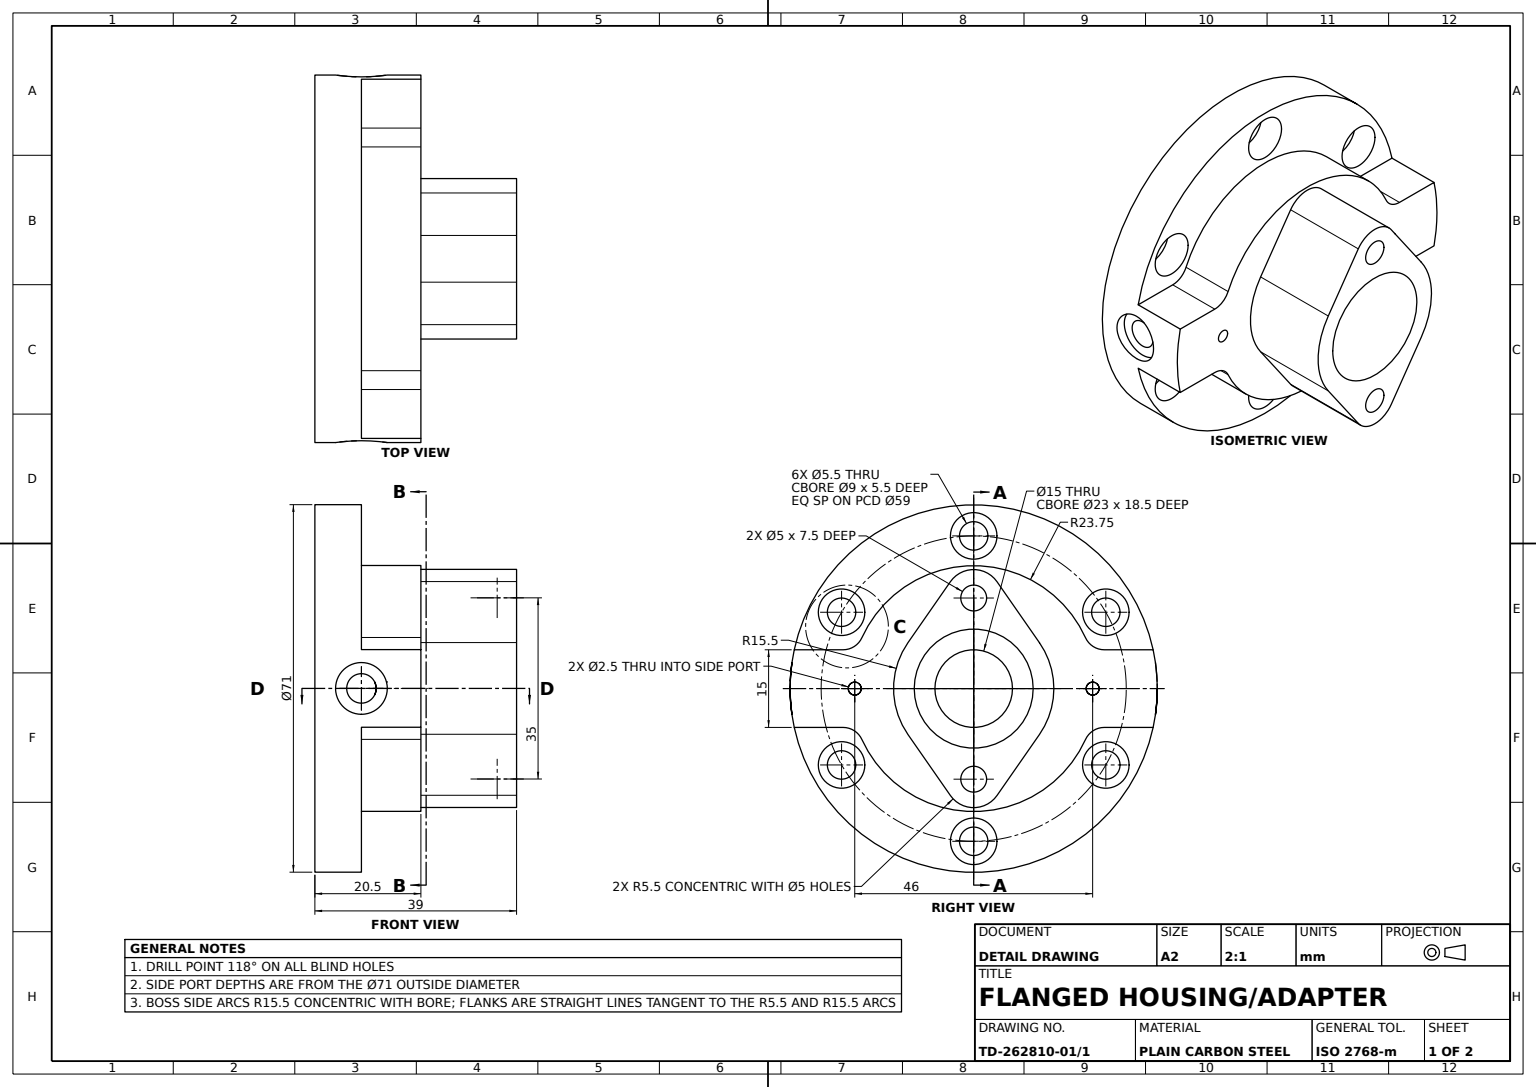
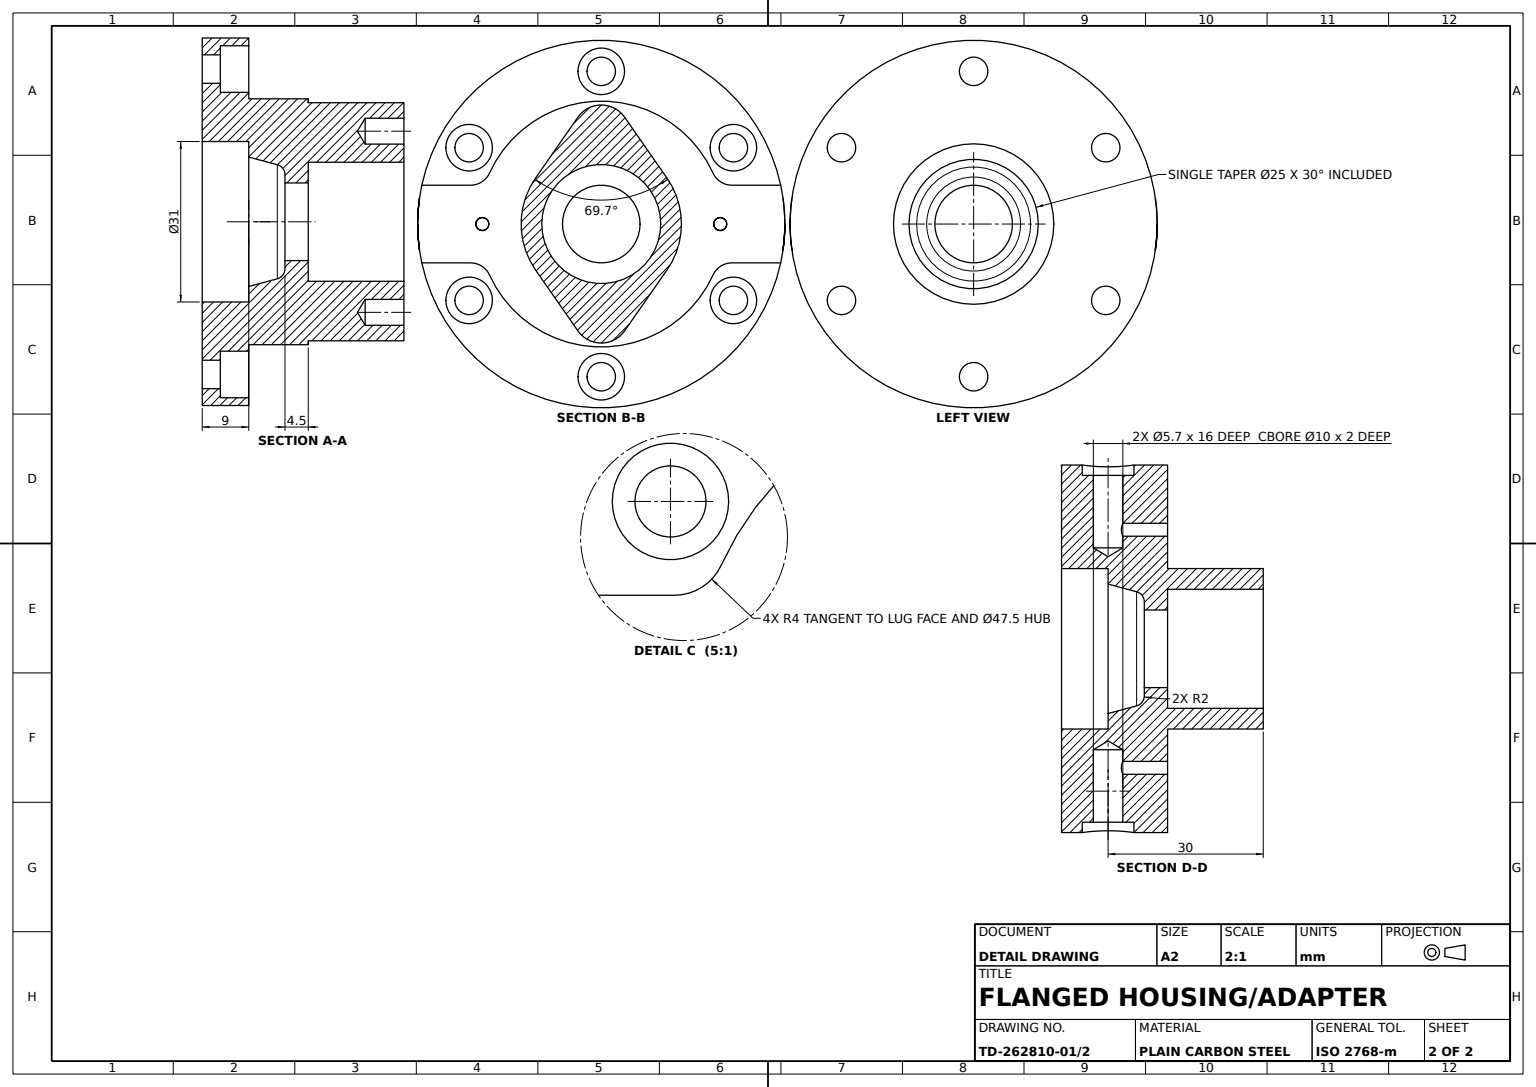
from build123d import *
from build123d.topology import SkipClean

# Parameters (mm, degrees)
SIDE_LUG_PROFILE_R                         = 7.5
SIDE_LUGS_DEPTH                            = 18.5
OVAL_MOUNTING_BOSS_DEPTH                   = 11.5
BOSS_EDGE_FILLET_R4_R                      = 4
FLANGE_HOLES_6X_C_BORE_5_5_D               = 5.5
FLANGE_HOLES_6X_C_BORE_5_5_CBORE_D         = 9
FLANGE_HOLES_6X_C_BORE_5_5_CBORE_DEPTH     = 5.5
SIDE_PORT_C_BORE_5_7_D                     = 5.7
SIDE_PORT_C_BORE_5_7_DEPTH                 = 16
SIDE_PORT_C_BORE_5_7_CBORE_D               = 10
SIDE_PORT_C_BORE_5_7_CBORE_DEPTH           = 2
SIDE_PORT_C_BORE_5_7_TIP                   = 1.712452764228547
SIDE_PORT_C_BORE_5_7_ON_FACE_2_D           = 5.7
SIDE_PORT_C_BORE_5_7_ON_FACE_2_DEPTH       = 16
SIDE_PORT_C_BORE_5_7_ON_FACE_2_CBORE_D     = 10
SIDE_PORT_C_BORE_5_7_ON_FACE_2_CBORE_DEPTH = 2
SIDE_PORT_C_BORE_5_7_ON_FACE_2_TIP         = 1.712452764228547
RELIEF_CUT_REACH                           = 56.229
RELIEF_CUT_END_RADIUS                      = 2.850000000000001
RELIEF_CUT_PROFILE_R                       = 1.250000000000001
RELIEF_CUT_PROFILE_R_2                     = 1.2500000000000009
LUG_DRILL_HOLES_5_D                        = 5
LUG_DRILL_HOLES_5_DEPTH                    = 7.5
LUG_DRILL_HOLES_5_TIP                      = 1.5021515475689007
BORE_EDGE_FILLET_R2_R                      = 2


with BuildPart() as part:
    # Flange Body Profile → Flange Body (revolve)
    with BuildSketch(Plane(origin=(0, 0, 0), x_dir=(0, 0, -1), z_dir=(1, 0, 0))):
        Polygon((15.5, 39), (15.500000000000002, 9), (12.5, 9), (10.624355652982135, 16), (7.5, 16), (7.5, 20.5), (11.5, 20.5), (11.5, 39), align=None)
        Polygon((35.5, 9.1e-16), (15.5, -2.45e-15), (15.500000000000002, 9), (35.5, 9.000000000000002), align=None)
    revolve(axis=Axis((0, 0, 0), (0, 1, 0)))

    # Side Lug Profile → Side Lugs (add)
    with SkipClean():  # the faces are left unmerged after this step: merging them gives an invalid solid
        with BuildSketch(Plane(origin=(0, 39, 0), x_dir=(1, 0, 0), z_dir=(0, 1, 0))):
            with BuildLine():
                Line((-20.642857142857142, 4.513584936565594), (-8.857142857142858, 12.720103003048491))
                ThreePointArc((-8.857142857142858, 12.720103003048491), (-2.49e-15, 15.499999999999995), (8.85714285714285, 12.720103003048491))
                Line((8.85714285714285, 12.720103003048491), (20.642857142857142, 4.513584936565599))
                ThreePointArc((20.642857142857142, 4.513584936565599), (23, 6.43e-15), (20.642857142857142, -4.513584936565586))
                Line((20.642857142857142, -4.513584936565586), (8.857142857142858, -12.720103003048482))
                ThreePointArc((8.857142857142858, -12.720103003048482), (9.5e-16, -15.499999999999996), (-8.857142857142854, -12.72010300304849))
                Line((-8.857142857142854, -12.72010300304849), (-20.642857142857142, -4.513584936565596))
                ThreePointArc((-20.642857142857142, -4.513584936565596), (-23, 6.7e-16), (-20.642857142857142, 4.513584936565594))
            make_face()
            with Locations(Location((0, 0, 0), (0, 0, 90))):
                Circle(SIDE_LUG_PROFILE_R, mode=Mode.SUBTRACT)
        extrude(amount=-SIDE_LUGS_DEPTH)

    # Oval Boss Profile → Oval Mounting Boss (add)
    with BuildSketch(Plane(origin=(0, 9.000000000000002, 0), x_dir=(1, 0, 0), z_dir=(0, 1, 0))):
        with BuildLine():
            Line((7.500000000000008, -34.69870314579495), (7.500000000000008, -22.534695471649933))
            ThreePointArc((7.500000000000008, -22.534695471649933), (23.750000000000004, 0), (7.500000000000008, 22.534695471649933))
            Line((7.500000000000008, 22.534695471649933), (7.500000000000008, 34.69870314579495))
            ThreePointArc((7.500000000000008, 34.69870314579495), (2.17e-15, 35.50000000000001), (-7.499999999999991, 34.69870314579495))
            Line((-7.499999999999991, 34.69870314579495), (-7.499999999999995, 22.534695471649936))
            ThreePointArc((-7.499999999999995, 22.534695471649936), (-23.75, 2.91e-15), (-7.499999999999995, -22.534695471649936))
            Line((-7.499999999999995, -22.534695471649936), (-7.499999999999991, -34.69870314579495))
            ThreePointArc((-7.499999999999991, -34.69870314579495), (2.17e-15, -35.50000000000001), (7.500000000000008, -34.69870314579495))
        make_face()
    extrude(amount=OVAL_MOUNTING_BOSS_DEPTH)

    # Boss Edge Fillet R4
    boss_edge_fillet_r4_edges = [part.edges().sort_by_distance(p)[0] for p in [
        (-7.499999999999995, 14.750000000000002, -22.534695471649933),
        (-7.499999999999998, 14.750000000000002, 22.534695471649936),
        (7.500000000000009, 14.750000000000002, 22.534695471649933),
        (7.500000000000007, 14.750000000000002, -22.534695471649933),
    ]]
    fillet(boss_edge_fillet_r4_edges, radius=BOSS_EDGE_FILLET_R4_R)

    # Flange Holes 6x C'bore Ø5.5 (through all)
    with Locations(Plane(origin=(0, 9.000000000000002, 0), x_dir=(1, 0, 0), z_dir=(0, 1, 0))):
        with Locations((-14.75, -25.547749412), (-29.5, 0), (-14.75, 25.547749412), (14.75, 25.547749412), (29.5, 0), (14.75, -25.547749412)):
            CounterBoreHole(FLANGE_HOLES_6X_C_BORE_5_5_D / 2, FLANGE_HOLES_6X_C_BORE_5_5_CBORE_D / 2, FLANGE_HOLES_6X_C_BORE_5_5_CBORE_DEPTH)

    # Side Port C'bore Ø5.7
    with Locations(Plane(origin=(0, 9, 35.5), x_dir=(1, 0, 0), z_dir=(0, 0, 1))):
        with Locations((0, 0)):
            CounterBoreHole(SIDE_PORT_C_BORE_5_7_D / 2, SIDE_PORT_C_BORE_5_7_CBORE_D / 2, SIDE_PORT_C_BORE_5_7_CBORE_DEPTH, depth=SIDE_PORT_C_BORE_5_7_DEPTH)
            with Locations((0, 0, -(SIDE_PORT_C_BORE_5_7_DEPTH + SIDE_PORT_C_BORE_5_7_TIP / 2))):  # 118° drill point
                Cone(0, SIDE_PORT_C_BORE_5_7_D / 2, SIDE_PORT_C_BORE_5_7_TIP, mode=Mode.SUBTRACT)

    # Side Port C'bore Ø5.7 on face 2
    with Locations(Plane(origin=(0, 9, -35.5), x_dir=(-1, 0, 0), z_dir=(0, 0, -1))):
        with Locations((0, 0)):
            CounterBoreHole(SIDE_PORT_C_BORE_5_7_ON_FACE_2_D / 2, SIDE_PORT_C_BORE_5_7_ON_FACE_2_CBORE_D / 2, SIDE_PORT_C_BORE_5_7_ON_FACE_2_CBORE_DEPTH, depth=SIDE_PORT_C_BORE_5_7_ON_FACE_2_DEPTH)
            with Locations((0, 0, -(SIDE_PORT_C_BORE_5_7_ON_FACE_2_DEPTH + SIDE_PORT_C_BORE_5_7_ON_FACE_2_TIP / 2))):  # 118° drill point
                Cone(0, SIDE_PORT_C_BORE_5_7_ON_FACE_2_D / 2, SIDE_PORT_C_BORE_5_7_ON_FACE_2_TIP, mode=Mode.SUBTRACT)

    # Relief Cut: up to this cylinder (the profile starts outside it)
    relief_cut_end = Plane(origin=(0, 9, 0), z_dir=(0, 0, -1)) * Cylinder(RELIEF_CUT_END_RADIUS, 165.158, mode=Mode.PRIVATE)
    # Relief Cut Profile → Relief Cut (cut, up to the surface)
    with BuildSketch(Plane(origin=(0, 20.5, 0), x_dir=(1, 0, 0), z_dir=(0, 1, 0)), mode=Mode.PRIVATE) as relief_cut_sk1:
        with Locations(Location((-8.24e-15, 23, 0), (0, 0, 270))):
            Circle(RELIEF_CUT_PROFILE_R)
    relief_cut_tool1 = extrude(relief_cut_sk1.sketch, amount=-RELIEF_CUT_REACH, mode=Mode.PRIVATE) - relief_cut_end
    add(relief_cut_tool1.solids().sort_by_distance((0, 20.5, -23))[0], mode=Mode.SUBTRACT)
    # Relief Cut Profile → Relief Cut (cut, up to the surface)
    with BuildSketch(Plane(origin=(0, 20.5, 0), x_dir=(1, 0, 0), z_dir=(0, 1, 0)), mode=Mode.PRIVATE) as relief_cut_sk2:
        with Locations(Location((5.64e-15, -23, 0), (0, 0, 270))):
            Circle(RELIEF_CUT_PROFILE_R_2)
    relief_cut_tool2 = extrude(relief_cut_sk2.sketch, amount=-RELIEF_CUT_REACH, mode=Mode.PRIVATE) - relief_cut_end
    add(relief_cut_tool2.solids().sort_by_distance((0, 20.5, 23))[0], mode=Mode.SUBTRACT)

    # Lug Drill Holes Ø5
    with Locations(Plane(origin=(0, 39, 0), x_dir=(1, 0, 0), z_dir=(0, 1, 0))):
        with Locations((-17.5, 0), (17.5, 0)):
            Hole(LUG_DRILL_HOLES_5_D / 2, depth=LUG_DRILL_HOLES_5_DEPTH)
            with Locations((0, 0, -(LUG_DRILL_HOLES_5_DEPTH + LUG_DRILL_HOLES_5_TIP / 2))):  # 118° drill point
                Cone(0, LUG_DRILL_HOLES_5_D / 2, LUG_DRILL_HOLES_5_TIP, mode=Mode.SUBTRACT)

    # Central Bore Profile → Central Bore (revolve, cut)
    with BuildSketch(Plane(origin=(0, 0, 0), x_dir=(0, 0, -1), z_dir=(1, 0, 0))):
        Polygon((12.5, 9), (0, 8.999999999999998), (0, 39), (11.5, 39), (11.5, 20.5), (7.5, 20.5), (7.5, 16), (10.624355652982135, 16), align=None)
    revolve(axis=Axis((0, 0, 0), (0, 1, 0)), mode=Mode.SUBTRACT)

    # Bore Edge Fillet R2
    bore_edge_fillet_r2_edges = [part.edges().sort_by_distance(p)[0] for p in [
        (-1.3e-15, 16, 10.624355652982135),
    ]]
    fillet(bore_edge_fillet_r2_edges, radius=BORE_EDGE_FILLET_R2_R)


solid = part.part
